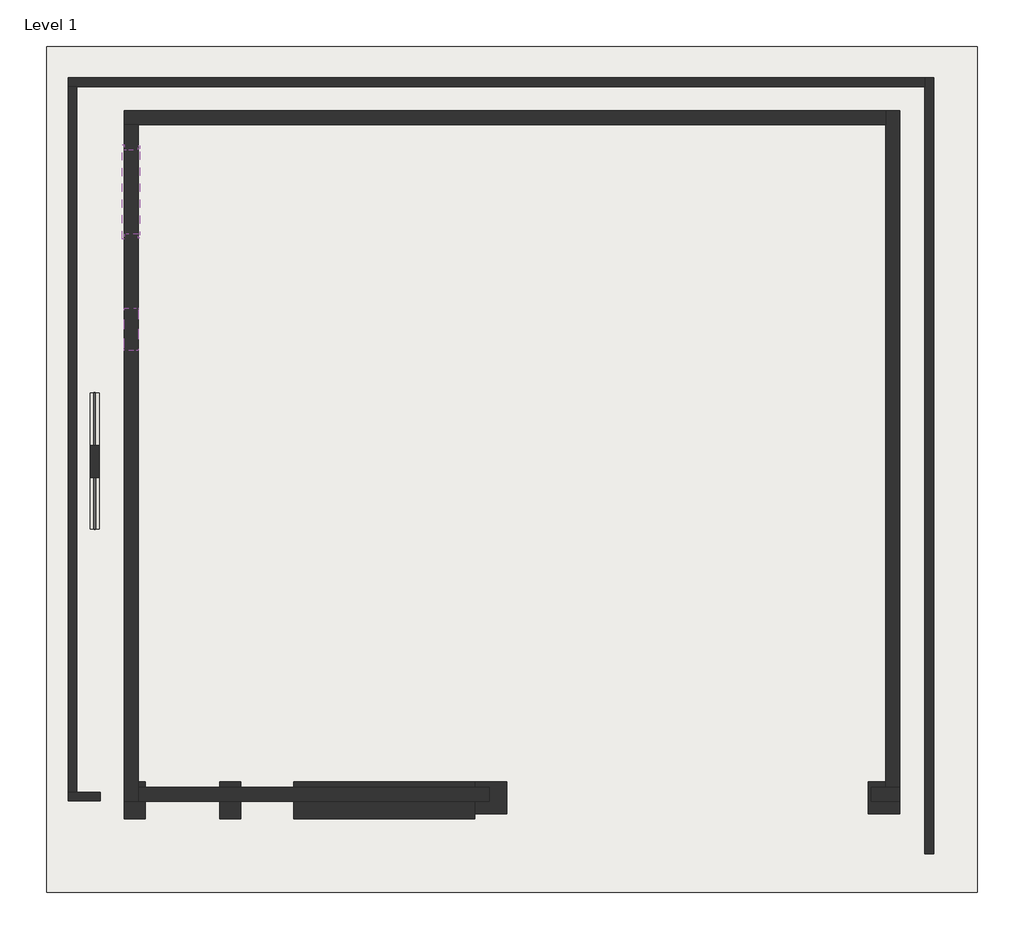
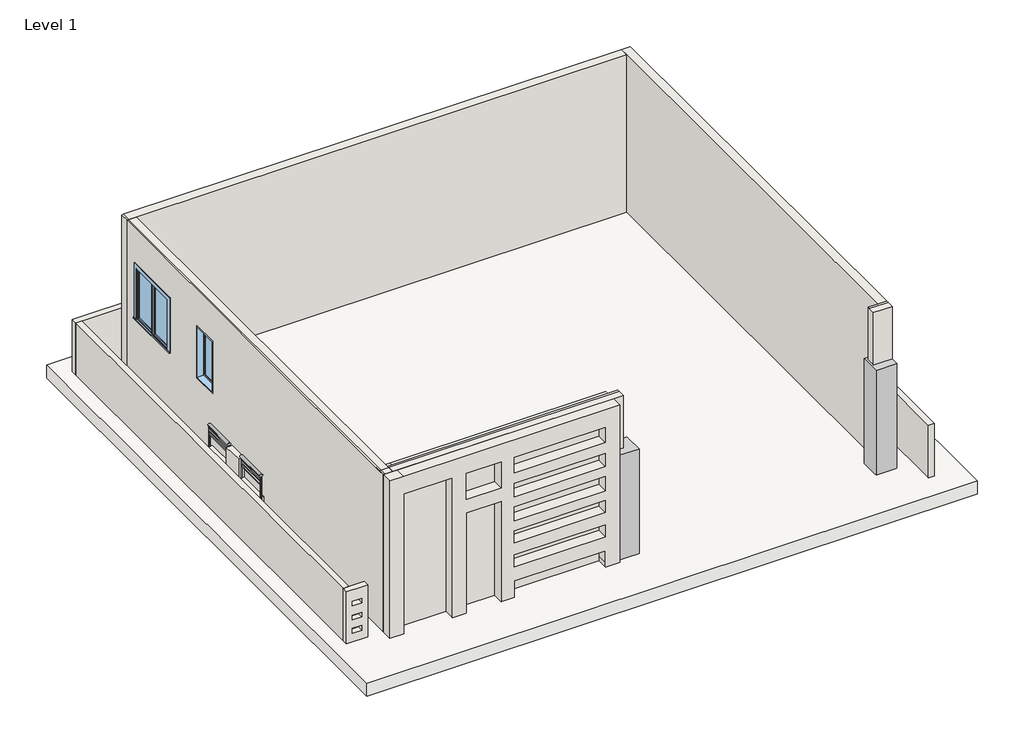
# One storey: 10 walls, 2 columns, 2 railings, 2 windows, 1 slab.
"""IFC4 building model written with IfcOpenShell, lengths in millimetres."""

from ifc_helpers import new_model, si_unit, point, frame, origin, origin_with_axes, place, context, project, spatial, polyline, ellipse_curve, trimmed, outline, extrude, faceted_brep, transform, mapped, element, save
from ifc_brep_helpers import plane_surface, extruded_surface, advanced_brep
from components import walls_6_walls_6_78742a1b, window_0862ab64, window_80bd9af0

model = new_model("IFC4")

# Units and contexts
model_context = context("Model", 3, world=origin())
ifc_project = project(units=[si_unit("LENGTHUNIT", "METRE", prefix="MILLI")], contexts=[model_context])

# Site, building, storey
site = spatial("IfcSite", under=ifc_project)
building = spatial("IfcBuilding", under=site)
storey = spatial("IfcBuildingStorey", under=building, Name="Level 1", Elevation=0.0)

# Columns
placement = place(None, origin())
element("IfcColumn", 1, ObjectType="Rectangular Column : 18\" x 18\"", at=placement, inside=storey, context=model_context, shape_type="SweptSolid", body=[
    extrude(outline(polyline([(1122.6002528, 1223.4609482), (665.4002528, 1223.4609482), (665.4002528, 1680.6609482), (919.4002528, 1680.6609482), (919.4002528, 1604.4609482), (710.3480866, 1604.4609482), (710.3480866, 1401.2609482), (1122.6002528, 1401.2609482), (1122.6002528, 1223.4609482)])), origin_with_axes(), (0.0, 0.0, 1.0), 2438.4),
])
element("IfcColumn", 2, ObjectType="Rectangular Column : 18\" x 18\"", at=placement, inside=storey, context=model_context, shape_type="SweptSolid", body=[
    extrude(outline(polyline([(-4541.5997472, 1680.6609482), (-4541.5997472, 1223.4609482), (-4998.7997472, 1223.4609482), (-4998.7997472, 1401.2609482), (-4789.9857575, 1401.2609482), (-4789.9857575, 1604.4609482), (-4998.7997472, 1604.4609482), (-4998.7997472, 1680.6609482), (-4541.5997472, 1680.6609482)])), origin_with_axes(), (0.0, 0.0, 1.0), 2438.4),
])

# Railings
element("IfcRailing", 3, ObjectType="Glass Panel - Bottom Fill", at=placement, inside=storey, context=model_context, shape_type="SolidModel", body=[
    advanced_brep(
    [(-10443.9247472, 7286.192958, 1402.0601563), (-10520.1247472, 7286.192958, 1402.0601562), (-10443.9247472, 6531.4144874, 1402.0601563), (-10520.1247472, 6531.4144874, 1402.0601563)],
    [
        (0, 1, ellipse_curve(frame((-10482.0247472, 7286.192958, 1402.0601563), z_axis=(0.0, 1.0, 0.0), x_axis=(-1.0, 0.0, 0.0)), 38.1, 28.575)),
        (1, 0, ellipse_curve(frame((-10482.0247472, 7286.192958, 1402.0601563), z_axis=(0.0, 1.0, 0.0), x_axis=(-1.0, 0.0, 0.0)), 38.1, 28.575)),
        (2, 3, ellipse_curve(frame((-10482.0247472, 6531.4144874, 1402.0601563), z_axis=(0.0, -1.0, 0.0), x_axis=(-1.0, 0.0, 0.0)), 38.1, 28.575)),
        (3, 2, ellipse_curve(frame((-10482.0247472, 6531.4144874, 1402.0601563), z_axis=(0.0, -1.0, 0.0), x_axis=(-1.0, 0.0, 0.0)), 38.1, 28.575)),
        (0, 2),
        (3, 1),
    ],
    [
        plane_surface(frame((-10482.0247472, 7286.192958, 1402.0601563), z_axis=(0.0, 1.0, 0.0), x_axis=(0.0, 0.0, -1.0))),
        plane_surface(frame((-10482.0247472, 6531.4144874, 1402.0601563), z_axis=(0.0, -1.0, 0.0), x_axis=(0.0, 0.0, -1.0))),
        extruded_surface(trimmed(ellipse_curve(frame((-10482.0247472, 6531.4144874, 1402.0601563), z_axis=(0.0, 1.0, 0.0), x_axis=(-1.0, 0.0, 0.0)), 38.1, 28.575), [point((-10443.9247472, 6531.4144874, 1402.0601563))], [point((-10520.1247472, 6531.4144874, 1402.0601562))], True, "CARTESIAN"), (0.0, 754.7784705999993, 0.0), 754.7784705999993),
        extruded_surface(trimmed(ellipse_curve(frame((-10482.0247472, 6531.4144874, 1402.0601563), z_axis=(0.0, 1.0, 0.0), x_axis=(-1.0, 0.0, 0.0)), 38.1, 28.575), [point((-10520.1247472, 6531.4144874, 1402.0601563))], [point((-10443.9247472, 6531.4144874, 1402.0601563))], True, "CARTESIAN"), (0.0, 754.7784705999993, 0.0), 754.7784705999993),
    ],
    [
        (0, [[1, 2]]),
        (1, [[3, 4]]),
        (2, [[-1, 5, -4, 6]]),
        (3, [[-2, -6, -3, -5]]),
    ],
),
    extrude(outline(polyline([(-10494.7247472, 7286.192958), (-10469.3247472, 7286.192958), (-10469.3247472, 6531.4144874), (-10494.7247472, 6531.4144874), (-10494.7247472, 7286.192958)])), frame((0.0, 0.0, 1287.7601563), z_axis=(0.0, 0.0, 1.0), x_axis=(1.0, 0.0, 0.0)), (0.0, 0.0, 1.0), 25.4),
    extrude(outline(polyline([(-10494.7247472, 7286.192958), (-10469.3247472, 7286.192958), (-10469.3247472, 6531.4144874), (-10494.7247472, 6531.4144874), (-10494.7247472, 7286.192958)])), frame((0.0, 0.0, 1186.1601563), z_axis=(0.0, 0.0, 1.0), x_axis=(1.0, 0.0, 0.0)), (0.0, 0.0, 1.0), 25.4),
    extrude(outline(polyline([(-10491.5497472, 6544.1144874), (-10472.4997472, 6544.1144874), (-10472.4997472, 6525.0644874), (-10491.5497472, 6525.0644874), (-10491.5497472, 6544.1144874)])), frame((0.0, 0.0, 487.6601563), z_axis=(0.0, 0.0, 1.0), x_axis=(1.0, 0.0, 0.0)), (0.0, 0.0, 1.0), 885.6788223),
    extrude(outline(polyline([(-10491.5497472, 7292.542958), (-10472.4997472, 7292.542958), (-10472.4997472, 7273.492958), (-10491.5497472, 7273.492958), (-10491.5497472, 7292.542958)])), frame((0.0, 0.0, 487.6601563), z_axis=(0.0, 0.0, 1.0), x_axis=(1.0, 0.0, 0.0)), (0.0, 0.0, 1.0), 885.6788223),
])
element("IfcRailing", 4, ObjectType="Glass Panel - Bottom Fill", at=placement, inside=storey, context=model_context, shape_type="SolidModel", body=[
    advanced_brep(
    [(-10437.5747472, 6074.2144874, 1402.0601563), (-10513.7747472, 6074.2144874, 1402.0601562), (-10437.5747472, 5330.392958, 1402.0601563), (-10513.7747472, 5330.392958, 1402.0601563)],
    [
        (0, 1, ellipse_curve(frame((-10475.6747472, 6074.2144874, 1402.0601563), z_axis=(0.0, 1.0, 0.0), x_axis=(-1.0, 0.0, 0.0)), 38.1, 28.575)),
        (1, 0, ellipse_curve(frame((-10475.6747472, 6074.2144874, 1402.0601563), z_axis=(0.0, 1.0, 0.0), x_axis=(-1.0, 0.0, 0.0)), 38.1, 28.575)),
        (2, 3, ellipse_curve(frame((-10475.6747472, 5330.392958, 1402.0601563), z_axis=(0.0, -1.0, 0.0), x_axis=(-1.0, 0.0, 0.0)), 38.1, 28.575)),
        (3, 2, ellipse_curve(frame((-10475.6747472, 5330.392958, 1402.0601563), z_axis=(0.0, -1.0, 0.0), x_axis=(-1.0, 0.0, 0.0)), 38.1, 28.575)),
        (0, 2),
        (3, 1),
    ],
    [
        plane_surface(frame((-10475.6747472, 6074.2144874, 1402.0601563), z_axis=(0.0, 1.0, 0.0), x_axis=(0.0, 0.0, -1.0))),
        plane_surface(frame((-10475.6747472, 5330.392958, 1402.0601563), z_axis=(0.0, -1.0, 0.0), x_axis=(0.0, 0.0, -1.0))),
        extruded_surface(trimmed(ellipse_curve(frame((-10475.6747472, 5330.392958, 1402.0601563), z_axis=(0.0, 1.0, 0.0), x_axis=(-1.0, 0.0, 0.0)), 38.1, 28.575), [point((-10437.5747472, 5330.392958, 1402.0601563))], [point((-10513.7747472, 5330.392958, 1402.0601562))], True, "CARTESIAN"), (0.0, 743.8215293999992, 0.0), 743.8215293999992),
        extruded_surface(trimmed(ellipse_curve(frame((-10475.6747472, 5330.392958, 1402.0601563), z_axis=(0.0, 1.0, 0.0), x_axis=(-1.0, 0.0, 0.0)), 38.1, 28.575), [point((-10513.7747472, 5330.392958, 1402.0601563))], [point((-10437.5747472, 5330.392958, 1402.0601563))], True, "CARTESIAN"), (0.0, 743.8215293999992, 0.0), 743.8215293999992),
    ],
    [
        (0, [[1, 2]]),
        (1, [[3, 4]]),
        (2, [[-1, 5, -4, 6]]),
        (3, [[-2, -6, -3, -5]]),
    ],
),
    extrude(outline(polyline([(-10488.3747472, 6074.2144874), (-10462.9747472, 6074.2144874), (-10462.9747472, 5330.392958), (-10488.3747472, 5330.392958), (-10488.3747472, 6074.2144874)])), frame((0.0, 0.0, 1287.7601563), z_axis=(0.0, 0.0, 1.0), x_axis=(1.0, 0.0, 0.0)), (0.0, 0.0, 1.0), 25.4),
    extrude(outline(polyline([(-10488.3747472, 6074.2144874), (-10462.9747472, 6074.2144874), (-10462.9747472, 5330.392958), (-10488.3747472, 5330.392958), (-10488.3747472, 6074.2144874)])), frame((0.0, 0.0, 1186.1601563), z_axis=(0.0, 0.0, 1.0), x_axis=(1.0, 0.0, 0.0)), (0.0, 0.0, 1.0), 25.4),
    extrude(outline(polyline([(-10485.1997472, 5343.092958), (-10466.1497472, 5343.092958), (-10466.1497472, 5324.042958), (-10485.1997472, 5324.042958), (-10485.1997472, 5343.092958)])), frame((0.0, 0.0, 487.6601563), z_axis=(0.0, 0.0, 1.0), x_axis=(1.0, 0.0, 0.0)), (0.0, 0.0, 1.0), 885.6788223),
    extrude(outline(polyline([(-10485.1997472, 6080.5644874), (-10466.1497472, 6080.5644874), (-10466.1497472, 6061.5144874), (-10485.1997472, 6061.5144874), (-10485.1997472, 6080.5644874)])), frame((0.0, 0.0, 487.6601563), z_axis=(0.0, 0.0, 1.0), x_axis=(1.0, 0.0, 0.0)), (0.0, 0.0, 1.0), 885.6788223),
])

# Slab
element("IfcSlab", 5, ObjectType="Generic - 12\"", at=placement, inside=storey, context=model_context, shape_type="SweptSolid", body=[
    extrude(outline(polyline([(2239.9566621, 12283.360814), (2239.9566621, 91.360814), (-11171.2433379, 91.360814), (-11171.2433379, 12283.360814), (2239.9566621, 12283.360814)])), frame((0.0, 0.0, -304.8), z_axis=(0.0, 0.0, 1.0), x_axis=(1.0, 0.0, 0.0)), (0.0, 0.0, 1.0), 304.8),
])

# Walls
element("IfcWall", 6, ObjectType="Generic - 5\"", at=placement, inside=storey, context=model_context, shape_type="SweptSolid", body=[
    extrude(outline(polyline([(7286.192958, -244.1613636), (5330.392958, -244.1613636), (5330.392958, 897.0632192), (6074.2144874, 897.0632192), (6074.2144874, 1354.2632192), (6531.4144874, 1354.2632192), (6531.4144874, 897.0632192), (7286.192958, 897.0632192), (7286.192958, -244.1613636)]), holes=[polyline([(6843.8232349, 512.7459623), (6843.8232349, 182.5459623), (7148.6232349, 182.5459623), (7148.6232349, 512.7459623), (6843.8232349, 512.7459623)]), polyline([(6361.2232349, 512.7459623), (6361.2232349, 182.5459623), (6666.0232349, 182.5459623), (6666.0232349, 512.7459623), (6361.2232349, 512.7459623)]), polyline([(5878.6232349, 512.7459623), (5878.6232349, 182.5459623), (6183.4232349, 182.5459623), (6183.4232349, 512.7459623), (5878.6232349, 512.7459623)]), polyline([(5421.4232349, 512.7459623), (5421.4232349, 182.5459623), (5726.2232349, 182.5459623), (5726.2232349, 512.7459623), (5421.4232349, 512.7459623)])]), frame((-10539.1747472, 0.0, 0.0), z_axis=(1.0, 0.0, 0.0), x_axis=(0.0, 1.0, 0.0)), (0.0, 0.0, 1.0), 127.0),
])
element("IfcWall", 7, ObjectType="Generic - 5\"", at=placement, inside=storey, context=model_context, shape_type="Brep", body=[
    faceted_brep([(-10861.0011236, 11706.6113669, 0.0), (-10734.0011236, 11706.6113669, 0.0), (1483.3988764, 11706.6113669, 0.0), (1483.3988764, 11706.6113669, 1219.2), (-10734.0011236, 11706.6113669, 1219.2), (-10861.0011236, 11706.6113669, 1219.2), (-10861.0011236, 11833.6113669, 0.0), (-10861.0011236, 11833.6113669, 1219.2), (1483.3988764, 11833.6113669, 1219.2), (1483.3988764, 11833.6113669, 0.0)], [[[0, 1, 2, 3, 4, 5]], [[6, 7, 8, 9]], [[2, 1, 0, 6, 9]], [[5, 4, 3, 8, 7]], [[0, 5, 7, 6]], [[3, 2, 9, 8]]]),
])
element("IfcWall", 8, ObjectType="Generic - 5\"", at=placement, inside=storey, context=model_context, shape_type="Brep", body=[
    faceted_brep([(-10734.0011236, 1535.0209854, 1219.2), (-10734.0011236, 1535.0209854, 949.3856619), (-10734.0011236, 1535.0209854, 843.1993865), (-10734.0011236, 1535.0209854, 622.3), (-10734.0011236, 1535.0209854, 512.7459623), (-10734.0011236, 1535.0209854, 321.7975209), (-10734.0011236, 1535.0209854, 201.1297196), (-10734.0011236, 1535.0209854, 0.0), (-10734.0011236, 11706.6113669, 0.0), (-10734.0011236, 11706.6113669, 1219.2), (-10861.0011236, 1535.0209854, 0.0), (-10861.0011236, 1535.0209854, 1213.0600738), (-10861.0011236, 1535.0209854, 1219.2), (-10861.0011236, 11706.6113669, 1219.2), (-10861.0011236, 11706.6113669, 0.0)], [[[0, 1, 2, 3, 4, 5, 6, 7, 8, 9]], [[10, 11, 12, 13, 14]], [[8, 7, 10, 14]], [[0, 9, 13, 12]], [[9, 8, 14, 13]], [[0, 12, 11, 10, 7, 6, 5, 4, 3, 2, 1]]]),
])
element("IfcWall", 9, ObjectType="Generic - 5\"", at=placement, inside=storey, context=model_context, shape_type="Brep", body=[
    faceted_brep([(1483.3988764, 11833.6113669, 0.0), (1483.3988764, 11706.6113669, 0.0), (1483.3988764, 644.9113669, 0.0), (1483.3988764, 644.9113669, 1219.2), (1483.3988764, 11706.6113669, 1219.2), (1483.3988764, 11833.6113669, 1219.2), (1610.3988764, 11833.6113669, 0.0), (1610.3988764, 11833.6113669, 1219.2), (1610.3988764, 644.9113669, 1219.2), (1610.3988764, 644.9113669, 0.0)], [[[0, 1, 2, 3, 4, 5]], [[6, 7, 8, 9]], [[2, 1, 0, 6, 9]], [[3, 2, 9, 8]], [[5, 4, 3, 8, 7]], [[0, 5, 7, 6]]]),
])
element("IfcWall", 10, ObjectType="Generic - 5\"", at=placement, inside=storey, context=model_context, shape_type="Brep", body=[
    faceted_brep([(-10861.0011236, 1408.0209854, 0.0), (-10397.0124309, 1408.0209854, 0.0), (-10397.0124309, 1408.0209854, 1213.0600738), (-10524.0124309, 1408.0209854, 1213.0600738), (-10861.0011236, 1408.0209854, 1213.0600738), (-10524.0124309, 1408.0209854, 949.3856619), (-10524.0124309, 1408.0209854, 843.1993865), (-10734.0011236, 1408.0209854, 843.1993865), (-10734.0011236, 1408.0209854, 949.3856619), (-10526.4747472, 1408.0209854, 622.3), (-10526.4747472, 1408.0209854, 512.7459623), (-10734.0011236, 1408.0209854, 512.7459623), (-10734.0011236, 1408.0209854, 622.3), (-10524.0124309, 1408.0209854, 321.7975209), (-10524.0124309, 1408.0209854, 201.1297196), (-10734.0011236, 1408.0209854, 201.1297196), (-10734.0011236, 1408.0209854, 321.7975209), (-10861.0011236, 1535.0209854, 0.0), (-10861.0011236, 1535.0209854, 1213.0600738), (-10524.0124309, 1535.0209854, 1213.0600738), (-10397.0124309, 1535.0209854, 1213.0600738), (-10397.0124309, 1535.0209854, 0.0), (-10524.0124309, 1535.0209854, 0.0), (-10734.0011236, 1535.0209854, 0.0), (-10524.0124309, 1535.0209854, 949.3856619), (-10734.0011236, 1535.0209854, 949.3856619), (-10734.0011236, 1535.0209854, 843.1993865), (-10524.0124309, 1535.0209854, 843.1993865), (-10526.4747472, 1535.0209854, 622.3), (-10734.0011236, 1535.0209854, 622.3), (-10734.0011236, 1535.0209854, 512.7459623), (-10526.4747472, 1535.0209854, 512.7459623), (-10524.0124309, 1535.0209854, 321.7975209), (-10734.0011236, 1535.0209854, 321.7975209), (-10734.0011236, 1535.0209854, 201.1297196), (-10524.0124309, 1535.0209854, 201.1297196)], [[[0, 1, 2, 3, 4], [5, 6, 7, 8], [9, 10, 11, 12], [13, 14, 15, 16]], [[17, 18, 19, 20, 21, 22, 23], [24, 25, 26, 27], [28, 29, 30, 31], [32, 33, 34, 35]], [[2, 1, 21, 20]], [[0, 4, 18, 17]], [[1, 0, 17, 23, 22, 21]], [[4, 3, 2, 20, 19, 18]], [[6, 5, 24, 27]], [[7, 6, 27, 26]], [[8, 7, 26, 25]], [[5, 8, 25, 24]], [[10, 9, 28, 31]], [[11, 10, 31, 30]], [[12, 11, 30, 29]], [[9, 12, 29, 28]], [[14, 13, 32, 35]], [[15, 14, 35, 34]], [[16, 15, 34, 33]], [[13, 16, 33, 32]]]),
])
element("IfcWall", 11, ObjectType="Generic - 8\"", at=placement, inside=storey, context=model_context, shape_type="Brep", body=[
    faceted_brep([(-10053.3997472, 11154.8609482, 0.0), (-9850.1997472, 11154.8609482, 0.0), (919.4002528, 11154.8609482, 0.0), (919.4002528, 11154.8609482, 3657.6), (-9850.1997472, 11154.8609482, 3657.6), (-10018.4747472, 11154.8609482, 3657.6), (-10053.3997472, 11154.8609482, 3657.6), (-10053.3997472, 11358.0609482, 0.0), (-10053.3997472, 11358.0609482, 3657.6), (-10018.4747472, 11358.0609482, 3657.6), (919.4002528, 11358.0609482, 3657.6), (919.4002528, 11358.0609482, 0.0)], [[[0, 1, 2, 3, 4, 5, 6]], [[7, 8, 9, 10, 11]], [[2, 1, 0, 7, 11]], [[0, 6, 8, 7]], [[3, 2, 11, 10]], [[6, 5, 9, 8]], [[5, 4, 3, 10, 9]]]),
])
element("IfcWall", 12, ObjectType="Generic - 8\"", at=placement, inside=storey, context=model_context, shape_type="Brep", body=[
    faceted_brep([(-9850.1997472, 1401.2609482, 0.0), (-9850.1997472, 1604.4609482, 0.0), (-9850.1997472, 11154.8609482, 0.0), (-9850.1997472, 11154.8609482, 3657.6), (-9850.1997472, 1604.4609482, 3657.6), (-9850.1997472, 1553.6609482, 3657.6), (-9850.1997472, 1401.2609482, 3657.6), (-9850.1997472, 10799.2609482, 2784.6136757), (-9850.1997472, 10799.2609482, 1565.4136757), (-9850.1997472, 9580.0609482, 1565.4136757), (-9850.1997472, 9580.0609482, 2784.6136757), (-9850.1997472, 7903.6609482, 2815.0771798), (-9850.1997472, 8513.2609482, 2815.0771798), (-9850.1997472, 8513.2609482, 1595.8771798), (-9850.1997472, 7903.6609482, 1595.8771798), (-10053.3997472, 1401.2609482, 0.0), (-10053.3997472, 1401.2609482, 3657.6), (-10053.3997472, 1553.6609482, 3657.6), (-10053.3997472, 11154.8609482, 3657.6), (-10053.3997472, 11154.8609482, 0.0), (-10053.3997472, 5306.9209854, 0.0), (-10053.3997472, 5179.9209854, 0.0), (-10053.3997472, 1535.0209854, 0.0), (-10053.3997472, 1408.0209854, 0.0), (-10053.3997472, 10799.2609482, 2784.6136757), (-10053.3997472, 9580.0609482, 2784.6136757), (-10053.3997472, 9580.0609482, 1565.4136757), (-10053.3997472, 10799.2609482, 1565.4136757), (-10053.3997472, 7903.6609482, 2815.0771798), (-10053.3997472, 7903.6609482, 1595.8771798), (-10053.3997472, 8513.2609482, 1595.8771798), (-10053.3997472, 8513.2609482, 2815.0771798), (-10019.8638097, 11154.8609482, 3657.6), (-10018.4747472, 11154.8609482, 3657.6), (-10018.4747472, 7286.192958, 3657.6), (-10018.4747472, 5317.692958, 3657.6), (-10018.4747472, 5144.9959854, 3657.6), (-10018.4747472, 1553.6609482, 3657.6), (-10018.4747472, 1401.2609482, 3657.6), (-10019.8638097, 1401.2609482, 3657.6), (-10019.8638097, 1553.6609482, 3657.6)], [[[0, 1, 2, 3, 4, 5, 6], [7, 8, 9, 10], [11, 12, 13, 14]], [[15, 16, 17, 18, 19, 20, 21, 22, 23], [24, 25, 26, 27], [28, 29, 30, 31]], [[2, 1, 0, 15, 23, 22, 21, 20, 19]], [[3, 2, 19, 18, 32, 33]], [[5, 4, 3, 33, 34, 35, 36, 37]], [[0, 6, 38, 39, 16, 15]], [[32, 18, 17, 40]], [[40, 17, 16, 39]], [[33, 32, 40, 37, 36, 35, 34]], [[6, 5, 37, 38]], [[37, 40, 39, 38]], [[8, 7, 24, 27]], [[9, 8, 27, 26]], [[10, 9, 26, 25]], [[7, 10, 25, 24]], [[29, 28, 11, 14]], [[30, 29, 14, 13]], [[31, 30, 13, 12]], [[28, 31, 12, 11]]]),
])
element("IfcWall", 13, ObjectType="Generic - 8\"", at=placement, inside=storey, context=model_context, shape_type="Brep", body=[
    faceted_brep([(-9850.1997472, 1604.4609482, 3657.6), (-4789.9857575, 1604.4609482, 3657.6), (-4789.9857575, 1604.4609482, 2438.4), (-4789.9857575, 1604.4609482, 0.0), (-4998.7997472, 1604.4609482, 0.0), (-9850.1997472, 1604.4609482, 0.0), (-9850.1997472, 1401.2609482, 3657.6), (-9850.1997472, 1401.2609482, 0.0), (-4998.7997472, 1401.2609482, 0.0), (-4789.9857575, 1401.2609482, 0.0), (-4789.9857575, 1401.2609482, 2438.4), (-4789.9857575, 1401.2609482, 3657.6), (-9850.1997472, 1553.6609482, 3657.6), (-4789.9857575, 1553.6609482, 3657.6)], [[[0, 1, 2, 3, 4, 5]], [[6, 7, 8, 9, 10, 11]], [[0, 5, 7, 6, 12]], [[3, 2, 1, 13, 11, 10, 9]], [[5, 4, 3, 9, 8, 7]], [[12, 6, 11, 13]], [[1, 0, 12, 13]]]),
    faceted_brep([(1122.6002528, 1604.4609482, 0.0), (919.4002528, 1604.4609482, 0.0), (710.3480866, 1604.4609482, 0.0), (710.3480866, 1604.4609482, 2438.4), (710.3480866, 1604.4609482, 3657.6), (919.4002528, 1604.4609482, 3657.6), (1122.6002528, 1604.4609482, 3657.6), (1122.6002528, 1401.2609482, 0.0), (1122.6002528, 1401.2609482, 2438.4), (1122.6002528, 1401.2609482, 3657.6), (710.3480866, 1401.2609482, 3657.6), (710.3480866, 1401.2609482, 2438.4), (710.3480866, 1401.2609482, 0.0), (1122.6002528, 1553.6609482, 3657.6), (710.3480866, 1553.6609482, 3657.6)], [[[0, 1, 2, 3, 4, 5, 6]], [[7, 8, 9, 10, 11, 12]], [[0, 6, 13, 9, 8, 7]], [[2, 1, 0, 7, 12]], [[4, 3, 2, 12, 11, 10, 14]], [[14, 10, 9, 13]], [[6, 5, 4, 14, 13]]]),
])
element("IfcWall", 14, ObjectType="Generic - 8\"", at=placement, inside=storey, context=model_context, shape_type="Brep", body=[
    faceted_brep([(919.4002528, 11358.0609482, 0.0), (919.4002528, 11154.8609482, 0.0), (919.4002528, 1680.6609482, 0.0), (919.4002528, 1604.4609482, 0.0), (919.4002528, 1604.4609482, 2438.4), (919.4002528, 1604.4609482, 3657.6), (919.4002528, 11154.8609482, 3657.6), (919.4002528, 11358.0609482, 3657.6), (1122.6002528, 11358.0609482, 0.0), (1122.6002528, 11358.0609482, 3657.6), (1122.6002528, 1604.4609482, 3657.6), (1122.6002528, 1604.4609482, 0.0)], [[[0, 1, 2, 3, 4, 5, 6, 7]], [[8, 9, 10, 11]], [[3, 2, 1, 0, 8, 11]], [[0, 7, 9, 8]], [[5, 4, 3, 11, 10]], [[7, 6, 5, 10, 9]]]),
])
walls_6_walls_6_shape = walls_6_walls_6_78742a1b(model_context)
element("IfcWall", 15, ObjectType="Walls 6 : Walls 6", at=placement, inside=storey, context=model_context, shape_type="MappedRepresentation", body=[
    mapped(walls_6_walls_6_shape, transform((0.0, 0.0, 0.0), x_axis=(1.0, 0.0, 0.0), y_axis=(0.0, 1.0, 0.0), z_axis=(0.0, 0.0, 1.0))),
])

# Windows
window_shape = window_0862ab64(model_context)
element("IfcWindow", 16, ObjectType="Casement Dbl with Trim : 48\" x 48\"", at=placement, inside=storey, context=model_context, shape_type="MappedRepresentation", body=[
    mapped(window_shape, transform((-9932.7497472, 10189.6609482, 651.0136757), x_axis=(0.0, 1.0, 0.0), y_axis=(-1.0, 0.0, 0.0), z_axis=(0.0, 0.0, 1.0))),
])
window_2_shape = window_80bd9af0(model_context)
element("IfcWindow", 17, ObjectType="Fixed : 24\" x 48\"", at=placement, inside=storey, context=model_context, shape_type="MappedRepresentation", body=[
    mapped(window_2_shape, transform((-9951.7997472, 8170.3609482, 681.4771798), x_axis=(0.0, -1.0, 0.0), y_axis=(1.0, 0.0, 0.0), z_axis=(0.0, 0.0, 1.0))),
])

save(model, "model.ifc")

# Revit data of these elements
# Type "Rectangular Column : 18\" x 18\""
#   Assembly Code = "B1010200"
#   Depth = 1' - 6"
#   Offset Base = 0' - 0"
#   Offset Top = 0' - 0"
#   Width = 1' - 6"
#   Material = none
# Type "Glass Panel - Bottom Fill"
#   Assembly Code = "C2010400"
#   built-in parameter 1008612 = 0.0416667 (stored number, unit not read)
#   built-in parameter 1008611 = 0.0416667 (stored number, unit not read)
#   built-in parameter 1008609 = 0.333333 (stored number, unit not read)
#   built-in parameter 1008604 = 0.166667 (stored number, unit not read)
#   built-in parameter 1008603 = 0.166667 (stored number, unit not read)
#   Railing Height = 3' - 0"
#   built-in parameter 1008630 = 2
#   built-in parameter 1008610 = 2
#   built-in parameter 1008618 = Baluster - Square : 3/4"
# Type "Generic - 12\""
#   Assembly Code = "B1010"
#   Function = 0
#   Layers, outside or top first: 1' - 0" no material (function 1)
# Type "Generic - 5\""
#   Assembly Code = "B2010"
#   Layers, outside or top first: 0' - 5" no material (function 1)
# Type "Generic - 8\""
#   Assembly Code = "B2010"
#   Layers, outside or top first: 0' - 8" no material (function 1)
# Type "Casement Dbl with Trim : 48\" x 48\""
#   Type Mark = "13"
#   Construction Type Id = "GSP4R"
#   Assembly Code = "B2020100"
#   Analytic Construction = "1/8 in Pilkington single glazing"
#   Visual Light Transmittance = 0.9
#   Thermal Resistance (R) = 1.53941 (h·ft²·°F)/BTU
#   Solar Heat Gain Coefficient = 0.78
#   Heat Transfer Coefficient (U) = 0.6496 BTU/(h·ft²·°F)
#   Height = 4' - 0"
#   Default Sill Height = 3' - 0"
#   Trim Projection - Ext. = 0' - 0 1/2"
#   Trim Projection - Int. = 0' - 0 3/4"
#   Trim Width - Exterior = 0' - 3 1/2"
#   Trim Width - Interior = 0' - 3 1/2"
#   Width = 4' - 0"
#   Window Inset = 0' - 0 3/4"
#   Define Thermal Properties by = 1
#   Glass Pane Material = Glass
#   Sash Material = Sash
#   Trim Exterior Material = Trim
#   Trim Interior Material = Trim
#   Wall Closure = (empty or 0)
# Type "Fixed : 24\" x 48\""
#   Type Mark = "2"
#   Construction Type Id = "GSP4R"
#   Assembly Code = "B2020100"
#   Analytic Construction = "1/8 in Pilkington single glazing"
#   Visual Light Transmittance = 0.9
#   Solar Heat Gain Coefficient = 0.78
#   Heat Transfer Coefficient (U) = 0.6496 BTU/(h·ft²·°F)
#   Height = 4' - 0"
#   Default Sill Height = 3' - 0"
#   Width = 2' - 0"
#   Window Inset = 0' - 0 3/4"
#   Define Thermal Properties by = 1
#   Glass Pane Material = Glass
#   Sash Material = Sash
#   Wall Closure = (empty or 0)
# Elements 1, 2 (IfcColumn, "Rectangular Column : 18\" x 18\"")
#   Phase Created = New Construction
#   Materials on its faces: "Default Wall"
# Elements 3, 4 (IfcRailing, "Glass Panel - Bottom Fill")
#   built-in parameter 1008621 = 1.59993 (stored number, unit not read)
#   Phase Created = New Construction
# Element 5 (IfcSlab, "Generic - 12\"")
#   Height Offset From Level = 0' - 0"
#   Phase Created = New Construction
#   Materials on its faces: "Default Floor"
# Element 6 (IfcWall, "Generic - 5\"")
#   built-in parameter 1001111 = -0' - 9.61265"
#   Top Offset = -7' - 6.68255"
#   Base Offset = -0' - 9.61265"
#   wall height = 5' - 2.9301"
#   Phase Created = New Construction
#   Base Constraint = Level 1
#   Top Constraint = Level 2
#   Materials on its faces: "Default Wall"
# Elements 7, 8, 9 (IfcWall, "Generic - 5\"")
#   Top Offset = -8' - 0"
#   Base Offset = 0' - 0"
#   wall height = 4' - 0"
#   Phase Created = New Construction
#   Base Constraint = Level 1
#   Top Constraint = Level 2
#   Materials on its faces: "Default Wall"
# Element 10 (IfcWall, "Generic - 5\"")
#   Top Offset = -8' - 0.24173"
#   Base Offset = 0' - 0"
#   wall height = 3' - 11.75827"
#   Phase Created = New Construction
#   Base Constraint = Level 1
#   Top Constraint = Level 2
#   Materials on its faces: "Default Wall"
# Elements 11, 12, 13, 14 (IfcWall, "Generic - 8\"")
#   Top Offset = 0' - 0"
#   Base Offset = 0' - 0"
#   Unconnected Height = 12' - 0"
#   wall height = 12' - 0"
#   Phase Created = New Construction
#   Base Constraint = Level 1
#   Materials on its faces: "Default Wall"
# Element 15 (IfcWall, "Walls 6 : Walls 6")
#   Phase Created = New Construction
#   Materials on its faces: "Default Wall"
# Element 16 (IfcWindow, "Casement Dbl with Trim : 48\" x 48\"")
#   Mark = "12"
#   Phase Created = New Construction
#   Materials on its faces: "Sash", "Trim", "Glass"
# Element 17 (IfcWindow, "Fixed : 24\" x 48\"")
#   Mark = "13"
#   Phase Created = New Construction
#   Materials on its faces: "Sash", "Glass"
# Materials
#   "Glass": class "Glass", colour RGB 0 128 192, transparency 0.75, Description = "Soda Lime Glass", Cost = 0
#   "Sash": class "Wood", colour RGB 224 178 126, transparency 0
#   "Trim": class "Wood", colour RGB 224 178 126, transparency 0
#   "Default Wall": colour RGB 128 128 128, transparency 0
#   "Default Floor": colour RGB 128 128 128, transparency 0
